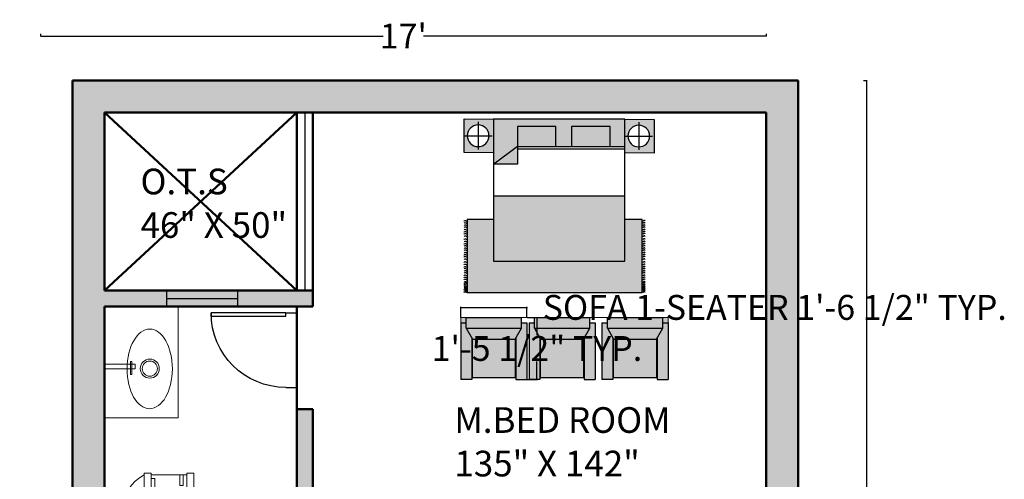
# Model space of a CAD drawing. Units: inches. Extents: x 679 to 1269, y 101 to 755.
# Tile 6 of 6: x 971 to 1248, y 626 to 755. Entities that reach past the tile are written whole.
import ezdxf

# ---------------------------------------------------------------- set-up
doc = ezdxf.new("R2010")
doc.units = ezdxf.units.IN
doc.header["$MEASUREMENT"] = 0
for name, color, linetype, lineweight in [('A-ANNO-DIMS', 2, 'Continuous', 18), ('A-AREA-IDEN', 7, 'Continuous', 25), ('A-DOOR', 4, 'Continuous', 25), ('A-FLOR-FIXT', 8, 'Continuous', 18), ('A-FURN', 32, 'Continuous', 18), ('A-FURN-PATT', 252, 'Continuous', 13), ('A-GLAZ', 4, 'Continuous', 25), ('A-WALL', 7, 'Continuous', 50), ('A-WALL-PATT', 8, 'Continuous', 13)]:
    doc.layers.add(name, color=color, linetype=linetype, lineweight=lineweight)
doc.layers.add('furniture', color=32, linetype='Continuous')
doc.styles.get("Standard").update_dxf_attribs({"font": 'arial.ttf'})
doc.dimstyles.get("Standard").update_dxf_attribs({"dimtxt": 7, "dimasz": 0.18, "dimexe": 0.18, "dimexo": 0.0625, "dimgap": 0.09, "dimtad": 0, "dimtih": 1, "dimtoh": 1, "dimzin": 0, "dimdsep": 46, "dimlunit": 3, "dimtxsty": 'Standard', "dimcen": 0.09, "dimadec": 0, "dimazin": 0, "dimtfac": 1, "dimtofl": 0, "dimtmove": 0, "dimatfit": 3, "dimfxl": 1, "dimtolj": 1, "dimtzin": 0, "dimarcsym": 0})

# ---------------------------------------------------------------- blocks, each defined once
blk = doc.blocks.new('*U4')
for p, q in [((0, 0), (0, -6)), ((40, 0), (40, -6))]:
    blk.add_line(p, q)
blk.add_lwpolyline([(0, 0), (0, 40), (1.75, 40), (1.75, 0)], close=True)
blk.add_arc((0, 0), 40, 0, 90)
blk = doc.blocks.new('CARPET')
at = {"layer": 'furniture'}
for p, q in [((-51.53, -98.11), (-51.53, -55.12)), ((-51.53, -55.12), (-41.27, -55.12)), ((36, -55.12), (51.55, -55.12)), ((51.55, -55.12), (51.55, -98.11)), ((51.55, -98.11), (-51.53, -98.11))]:
    blk.add_line(p, q, dxfattribs=at)
for points, knots in [([(-53.37, -55.99), (-53.22, -55.8), (-52.9, -55.41), (-52.34, -55.8), (-51.89, -56.08), (-51.65, -55.91), (-51.53, -55.83)], [0, 0, 0, 0, 0.653278, 1.290138, 1.740457, 2.114451, 2.114451, 2.114451, 2.114451]), ([(-53.37, -57.26), (-53.22, -57.07), (-52.9, -56.67), (-52.34, -57.07), (-51.89, -57.35), (-51.65, -57.17), (-51.53, -57.1)], [0, 0, 0, 0, 0.653278, 1.290138, 1.740457, 2.114451, 2.114451, 2.114451, 2.114451]), ([(53.37, -55.99), (53.22, -55.8), (52.9, -55.41), (52.34, -55.8), (51.89, -56.08), (51.65, -55.91), (51.53, -55.83)], [0, 0, 0, 0, 0.653278, 1.290138, 1.740457, 2.114451, 2.114451, 2.114451, 2.114451]), ([(53.37, -57.26), (53.22, -57.07), (52.9, -56.67), (52.34, -57.07), (51.89, -57.35), (51.65, -57.17), (51.53, -57.1)], [0, 0, 0, 0, 0.653278, 1.290138, 1.740457, 2.114451, 2.114451, 2.114451, 2.114451]), ([(-53.37, -58.59), (-53.22, -58.4), (-52.9, -58.01), (-52.34, -58.4), (-51.89, -58.68), (-51.65, -58.5), (-51.53, -58.43)], [0, 0, 0, 0, 0.653278, 1.290138, 1.740457, 2.114451, 2.114451, 2.114451, 2.114451]), ([(-53.37, -59.78), (-53.22, -59.58), (-52.9, -59.19), (-52.34, -59.58), (-51.89, -59.86), (-51.65, -59.69), (-51.53, -59.61)], [0, 0, 0, 0, 0.653278, 1.290138, 1.740457, 2.114451, 2.114451, 2.114451, 2.114451]), ([(-53.37, -61.22), (-53.22, -61.02), (-52.9, -60.63), (-52.34, -61.02), (-51.89, -61.3), (-51.65, -61.13), (-51.53, -61.05)], [0, 0, 0, 0, 0.653278, 1.290138, 1.740457, 2.114451, 2.114451, 2.114451, 2.114451]), ([(-53.37, -62.44), (-53.22, -62.25), (-52.9, -61.86), (-52.34, -62.25), (-51.89, -62.53), (-51.65, -62.36), (-51.53, -62.28)], [0, 0, 0, 0, 0.653278, 1.290138, 1.740457, 2.114451, 2.114451, 2.114451, 2.114451]), ([(-53.37, -63.63), (-53.22, -63.43), (-52.9, -63.04), (-52.34, -63.43), (-51.89, -63.72), (-51.65, -63.54), (-51.53, -63.46)], [0, 0, 0, 0, 0.653278, 1.290138, 1.740457, 2.114451, 2.114451, 2.114451, 2.114451]), ([(53.37, -58.59), (53.22, -58.4), (52.9, -58.01), (52.34, -58.4), (51.89, -58.68), (51.65, -58.5), (51.53, -58.43)], [0, 0, 0, 0, 0.653278, 1.290138, 1.740457, 2.114451, 2.114451, 2.114451, 2.114451]), ([(53.37, -59.78), (53.22, -59.58), (52.9, -59.19), (52.34, -59.58), (51.89, -59.86), (51.65, -59.69), (51.53, -59.61)], [0, 0, 0, 0, 0.653278, 1.290138, 1.740457, 2.114451, 2.114451, 2.114451, 2.114451]), ([(53.37, -61.22), (53.22, -61.02), (52.9, -60.63), (52.34, -61.02), (51.89, -61.3), (51.65, -61.13), (51.53, -61.05)], [0, 0, 0, 0, 0.653278, 1.290138, 1.740457, 2.114451, 2.114451, 2.114451, 2.114451]), ([(53.37, -62.44), (53.22, -62.25), (52.9, -61.86), (52.34, -62.25), (51.89, -62.53), (51.65, -62.36), (51.53, -62.28)], [0, 0, 0, 0, 0.653278, 1.290138, 1.740457, 2.114451, 2.114451, 2.114451, 2.114451]), ([(53.37, -63.63), (53.22, -63.43), (52.9, -63.04), (52.34, -63.43), (51.89, -63.72), (51.65, -63.54), (51.53, -63.46)], [0, 0, 0, 0, 0.653278, 1.290138, 1.740457, 2.114451, 2.114451, 2.114451, 2.114451]), ([(-53.37, -65.07), (-53.22, -64.87), (-52.9, -64.48), (-52.34, -64.87), (-51.89, -65.15), (-51.65, -64.98), (-51.53, -64.9)], [0, 0, 0, 0, 0.653278, 1.290138, 1.740457, 2.114451, 2.114451, 2.114451, 2.114451]), ([(-53.37, -66.76), (-53.22, -66.56), (-52.9, -66.17), (-52.34, -66.56), (-51.89, -66.84), (-51.65, -66.67), (-51.53, -66.59)], [0, 0, 0, 0, 0.653278, 1.290138, 1.740457, 2.114451, 2.114451, 2.114451, 2.114451]), ([(-53.37, -68.2), (-53.22, -68), (-52.9, -67.61), (-52.34, -68), (-51.89, -68.28), (-51.65, -68.11), (-51.53, -68.03)], [0, 0, 0, 0, 0.653278, 1.290138, 1.740457, 2.114451, 2.114451, 2.114451, 2.114451]), ([(-53.37, -69.53), (-53.22, -69.33), (-52.9, -68.94), (-52.34, -69.33), (-51.89, -69.61), (-51.65, -69.44), (-51.53, -69.36)], [0, 0, 0, 0, 0.653278, 1.290138, 1.740457, 2.114451, 2.114451, 2.114451, 2.114451]), ([(53.37, -65.07), (53.22, -64.87), (52.9, -64.48), (52.34, -64.87), (51.89, -65.15), (51.65, -64.98), (51.53, -64.9)], [0, 0, 0, 0, 0.653278, 1.290138, 1.740457, 2.114451, 2.114451, 2.114451, 2.114451]), ([(53.37, -66.76), (53.22, -66.56), (52.9, -66.17), (52.34, -66.56), (51.89, -66.84), (51.65, -66.67), (51.53, -66.59)], [0, 0, 0, 0, 0.653278, 1.290138, 1.740457, 2.114451, 2.114451, 2.114451, 2.114451]), ([(53.37, -68.2), (53.22, -68), (52.9, -67.61), (52.34, -68), (51.89, -68.28), (51.65, -68.11), (51.53, -68.03)], [0, 0, 0, 0, 0.653278, 1.290138, 1.740457, 2.114451, 2.114451, 2.114451, 2.114451]), ([(53.37, -69.53), (53.22, -69.33), (52.9, -68.94), (52.34, -69.33), (51.89, -69.61), (51.65, -69.44), (51.53, -69.36)], [0, 0, 0, 0, 0.653278, 1.290138, 1.740457, 2.114451, 2.114451, 2.114451, 2.114451]), ([(-53.37, -70.79), (-53.22, -70.6), (-52.9, -70.21), (-52.34, -70.6), (-51.89, -70.88), (-51.65, -70.7), (-51.53, -70.63)], [0, 0, 0, 0, 0.653278, 1.290138, 1.740457, 2.114451, 2.114451, 2.114451, 2.114451]), ([(-53.37, -72.12), (-53.22, -71.93), (-52.9, -71.54), (-52.34, -71.93), (-51.89, -72.21), (-51.65, -72.04), (-51.53, -71.96)], [0, 0, 0, 0, 0.653278, 1.290138, 1.740457, 2.114451, 2.114451, 2.114451, 2.114451]), ([(-53.37, -73.31), (-53.22, -73.11), (-52.9, -72.72), (-52.34, -73.11), (-51.89, -73.4), (-51.65, -73.22), (-51.53, -73.14)], [0, 0, 0, 0, 0.653278, 1.290138, 1.740457, 2.114451, 2.114451, 2.114451, 2.114451]), ([(-53.37, -74.75), (-53.22, -74.55), (-52.9, -74.16), (-52.34, -74.55), (-51.89, -74.83), (-51.65, -74.66), (-51.53, -74.58)], [0, 0, 0, 0, 0.653278, 1.290138, 1.740457, 2.114451, 2.114451, 2.114451, 2.114451]), ([(53.37, -70.79), (53.22, -70.6), (52.9, -70.21), (52.34, -70.6), (51.89, -70.88), (51.65, -70.7), (51.53, -70.63)], [0, 0, 0, 0, 0.653278, 1.290138, 1.740457, 2.114451, 2.114451, 2.114451, 2.114451]), ([(53.37, -72.12), (53.22, -71.93), (52.9, -71.54), (52.34, -71.93), (51.89, -72.21), (51.65, -72.04), (51.53, -71.96)], [0, 0, 0, 0, 0.653278, 1.290138, 1.740457, 2.114451, 2.114451, 2.114451, 2.114451]), ([(53.37, -73.31), (53.22, -73.11), (52.9, -72.72), (52.34, -73.11), (51.89, -73.4), (51.65, -73.22), (51.53, -73.14)], [0, 0, 0, 0, 0.653278, 1.290138, 1.740457, 2.114451, 2.114451, 2.114451, 2.114451]), ([(53.37, -74.75), (53.22, -74.55), (52.9, -74.16), (52.34, -74.55), (51.89, -74.83), (51.65, -74.66), (51.53, -74.58)], [0, 0, 0, 0, 0.653278, 1.290138, 1.740457, 2.114451, 2.114451, 2.114451, 2.114451]), ([(-53.37, -75.98), (-53.22, -75.78), (-52.9, -75.39), (-52.34, -75.78), (-51.89, -76.06), (-51.65, -75.89), (-51.53, -75.81)], [0, 0, 0, 0, 0.653278, 1.290138, 1.740457, 2.114451, 2.114451, 2.114451, 2.114451]), ([(-53.37, -77.16), (-53.22, -76.96), (-52.9, -76.57), (-52.34, -76.96), (-51.89, -77.25), (-51.65, -77.07), (-51.53, -76.99)], [0, 0, 0, 0, 0.653278, 1.290138, 1.740457, 2.114451, 2.114451, 2.114451, 2.114451]), ([(-53.37, -78.6), (-53.22, -78.4), (-52.9, -78.01), (-52.34, -78.4), (-51.89, -78.68), (-51.65, -78.51), (-51.53, -78.43)], [0, 0, 0, 0, 0.653278, 1.290138, 1.740457, 2.114451, 2.114451, 2.114451, 2.114451]), ([(-53.37, -80.29), (-53.22, -80.09), (-52.9, -79.7), (-52.34, -80.09), (-51.89, -80.37), (-51.65, -80.2), (-51.53, -80.12)], [0, 0, 0, 0, 0.653278, 1.290138, 1.740457, 2.114451, 2.114451, 2.114451, 2.114451]), ([(53.37, -75.98), (53.22, -75.78), (52.9, -75.39), (52.34, -75.78), (51.89, -76.06), (51.65, -75.89), (51.53, -75.81)], [0, 0, 0, 0, 0.653278, 1.290138, 1.740457, 2.114451, 2.114451, 2.114451, 2.114451]), ([(53.37, -77.16), (53.22, -76.96), (52.9, -76.57), (52.34, -76.96), (51.89, -77.25), (51.65, -77.07), (51.53, -76.99)], [0, 0, 0, 0, 0.653278, 1.290138, 1.740457, 2.114451, 2.114451, 2.114451, 2.114451]), ([(53.37, -78.6), (53.22, -78.4), (52.9, -78.01), (52.34, -78.4), (51.89, -78.68), (51.65, -78.51), (51.53, -78.43)], [0, 0, 0, 0, 0.653278, 1.290138, 1.740457, 2.114451, 2.114451, 2.114451, 2.114451]), ([(53.37, -80.29), (53.22, -80.09), (52.9, -79.7), (52.34, -80.09), (51.89, -80.37), (51.65, -80.2), (51.53, -80.12)], [0, 0, 0, 0, 0.653278, 1.290138, 1.740457, 2.114451, 2.114451, 2.114451, 2.114451]), ([(-53.37, -81.73), (-53.22, -81.53), (-52.9, -81.14), (-52.34, -81.53), (-51.89, -81.81), (-51.65, -81.64), (-51.53, -81.56)], [0, 0, 0, 0, 0.653278, 1.290138, 1.740457, 2.114451, 2.114451, 2.114451, 2.114451]), ([(-53.37, -83.06), (-53.22, -82.86), (-52.9, -82.47), (-52.34, -82.86), (-51.89, -83.14), (-51.65, -82.97), (-51.53, -82.89)], [0, 0, 0, 0, 0.653278, 1.290138, 1.740457, 2.114451, 2.114451, 2.114451, 2.114451]), ([(-53.37, -84.18), (-53.22, -83.99), (-52.9, -83.6), (-52.34, -83.99), (-51.89, -84.27), (-51.65, -84.09), (-51.53, -84.02)], [0, 0, 0, 0, 0.653278, 1.290138, 1.740457, 2.114451, 2.114451, 2.114451, 2.114451]), ([(-53.37, -85.51), (-53.22, -85.32), (-52.9, -84.93), (-52.34, -85.32), (-51.89, -85.6), (-51.65, -85.42), (-51.53, -85.35)], [0, 0, 0, 0, 0.653278, 1.290138, 1.740457, 2.114451, 2.114451, 2.114451, 2.114451]), ([(-53.37, -86.7), (-53.22, -86.5), (-52.9, -86.11), (-52.34, -86.5), (-51.89, -86.78), (-51.65, -86.61), (-51.53, -86.53)], [0, 0, 0, 0, 0.653278, 1.290138, 1.740457, 2.114451, 2.114451, 2.114451, 2.114451]), ([(53.37, -81.73), (53.22, -81.53), (52.9, -81.14), (52.34, -81.53), (51.89, -81.81), (51.65, -81.64), (51.53, -81.56)], [0, 0, 0, 0, 0.653278, 1.290138, 1.740457, 2.114451, 2.114451, 2.114451, 2.114451]), ([(53.37, -83.06), (53.22, -82.86), (52.9, -82.47), (52.34, -82.86), (51.89, -83.14), (51.65, -82.97), (51.53, -82.89)], [0, 0, 0, 0, 0.653278, 1.290138, 1.740457, 2.114451, 2.114451, 2.114451, 2.114451]), ([(53.37, -84.18), (53.22, -83.99), (52.9, -83.6), (52.34, -83.99), (51.89, -84.27), (51.65, -84.09), (51.53, -84.02)], [0, 0, 0, 0, 0.653278, 1.290138, 1.740457, 2.114451, 2.114451, 2.114451, 2.114451]), ([(53.37, -85.51), (53.22, -85.32), (52.9, -84.93), (52.34, -85.32), (51.89, -85.6), (51.65, -85.42), (51.53, -85.35)], [0, 0, 0, 0, 0.653278, 1.290138, 1.740457, 2.114451, 2.114451, 2.114451, 2.114451]), ([(53.37, -86.7), (53.22, -86.5), (52.9, -86.11), (52.34, -86.5), (51.89, -86.78), (51.65, -86.61), (51.53, -86.53)], [0, 0, 0, 0, 0.653278, 1.290138, 1.740457, 2.114451, 2.114451, 2.114451, 2.114451]), ([(-53.37, -88.14), (-53.22, -87.94), (-52.9, -87.55), (-52.34, -87.94), (-51.89, -88.22), (-51.65, -88.05), (-51.53, -87.97)], [0, 0, 0, 0, 0.653278, 1.290138, 1.740457, 2.114451, 2.114451, 2.114451, 2.114451]), ([(-53.37, -89.36), (-53.22, -89.17), (-52.9, -88.78), (-52.34, -89.17), (-51.89, -89.45), (-51.65, -89.28), (-51.53, -89.2)], [0, 0, 0, 0, 0.653278, 1.290138, 1.740457, 2.114451, 2.114451, 2.114451, 2.114451]), ([(-53.37, -90.55), (-53.22, -90.35), (-52.9, -89.96), (-52.34, -90.35), (-51.89, -90.64), (-51.65, -90.46), (-51.53, -90.38)], [0, 0, 0, 0, 0.653278, 1.290138, 1.740457, 2.114451, 2.114451, 2.114451, 2.114451]), ([(-53.37, -91.99), (-53.22, -91.79), (-52.9, -91.4), (-52.34, -91.79), (-51.89, -92.07), (-51.65, -91.9), (-51.53, -91.82)], [0, 0, 0, 0, 0.653278, 1.290138, 1.740457, 2.114451, 2.114451, 2.114451, 2.114451]), ([(-53.37, -92.69), (-53.22, -92.48), (-52.9, -92.08), (-52.35, -92.49), (-51.89, -92.77), (-51.65, -92.6), (-51.53, -92.52)], [0, 0, 0, 0, 0.663904, 1.307406, 1.757725, 2.131719, 2.131719, 2.131719, 2.131719]), ([(53.37, -88.14), (53.22, -87.94), (52.9, -87.55), (52.34, -87.94), (51.89, -88.22), (51.65, -88.05), (51.53, -87.97)], [0, 0, 0, 0, 0.653278, 1.290138, 1.740457, 2.114451, 2.114451, 2.114451, 2.114451]), ([(53.37, -89.36), (53.22, -89.17), (52.9, -88.78), (52.34, -89.17), (51.89, -89.45), (51.65, -89.28), (51.53, -89.2)], [0, 0, 0, 0, 0.653278, 1.290138, 1.740457, 2.114451, 2.114451, 2.114451, 2.114451]), ([(53.37, -90.55), (53.22, -90.35), (52.9, -89.96), (52.34, -90.35), (51.9, -90.63), (51.66, -90.47), (51.55, -90.4)], [0, 0, 0, 0, 0.653278, 1.290138, 1.740457, 2.0926, 2.0926, 2.0926, 2.0926]), ([(53.37, -91.99), (53.22, -91.79), (52.9, -91.4), (52.34, -91.79), (51.9, -92.07), (51.66, -91.91), (51.55, -91.83)], [0, 0, 0, 0, 0.653278, 1.290138, 1.740457, 2.0926, 2.0926, 2.0926, 2.0926]), ([(53.37, -92.69), (53.22, -92.49), (52.9, -92.09), (52.34, -92.49), (51.9, -92.77), (51.66, -92.61), (51.55, -92.53)], [0, 0, 0, 0, 0.656792, 1.295826, 1.746145, 2.098292, 2.098292, 2.098292, 2.098292]), ([(-53.37, -93.61), (-53.22, -93.42), (-52.9, -93.03), (-52.34, -93.42), (-51.89, -93.7), (-51.65, -93.52), (-51.53, -93.45)], [0, 0, 0, 0, 0.653278, 1.290138, 1.740457, 2.114451, 2.114451, 2.114451, 2.114451]), ([(-53.37, -94.55), (-53.22, -94.35), (-52.9, -93.96), (-52.34, -94.35), (-51.89, -94.63), (-51.65, -94.46), (-51.53, -94.38)], [0, 0, 0, 0, 0.653278, 1.290138, 1.740457, 2.114451, 2.114451, 2.114451, 2.114451]), ([(-53.37, -95.05), (-53.22, -94.85), (-52.9, -94.46), (-52.34, -94.85), (-51.89, -95.14), (-51.65, -94.96), (-51.53, -94.88)], [0, 0, 0, 0, 0.653278, 1.290138, 1.740457, 2.114451, 2.114451, 2.114451, 2.114451]), ([(-53.37, -95.73), (-53.22, -95.54), (-52.9, -95.15), (-52.34, -95.54), (-51.89, -95.82), (-51.65, -95.65), (-51.53, -95.57)], [0, 0, 0, 0, 0.653278, 1.290138, 1.740457, 2.114451, 2.114451, 2.114451, 2.114451]), ([(-53.37, -96.38), (-53.22, -96.18), (-52.9, -95.79), (-52.34, -96.18), (-51.89, -96.47), (-51.65, -96.29), (-51.53, -96.21)], [0, 0, 0, 0, 0.653278, 1.290138, 1.740457, 2.114451, 2.114451, 2.114451, 2.114451]), ([(-53.37, -97.17), (-53.22, -96.98), (-52.9, -96.59), (-52.34, -96.98), (-51.89, -97.26), (-51.65, -97.08), (-51.53, -97.01)], [0, 0, 0, 0, 0.653278, 1.290138, 1.740457, 2.114451, 2.114451, 2.114451, 2.114451]), ([(-53.37, -97.99), (-53.22, -97.79), (-52.9, -97.4), (-52.34, -97.79), (-51.89, -98.08), (-51.65, -97.9), (-51.53, -97.82)], [0, 0, 0, 0, 0.653278, 1.290138, 1.740457, 2.114451, 2.114451, 2.114451, 2.114451]), ([(53.37, -95.78), (53.22, -95.58), (52.9, -95.19), (52.34, -95.58), (51.89, -95.86), (51.65, -95.69), (51.53, -95.61)], [0, 0, 0, 0, 0.653278, 1.290138, 1.740457, 2.114451, 2.114451, 2.114451, 2.114451]), ([(53.37, -96.43), (53.22, -96.23), (52.9, -95.84), (52.34, -96.23), (51.89, -96.51), (51.65, -96.34), (51.53, -96.26)], [0, 0, 0, 0, 0.653278, 1.290138, 1.740457, 2.114451, 2.114451, 2.114451, 2.114451]), ([(53.37, -97.22), (53.22, -97.02), (52.9, -96.63), (52.34, -97.02), (51.89, -97.3), (51.65, -97.13), (51.53, -97.05)], [0, 0, 0, 0, 0.653278, 1.290138, 1.740457, 2.114451, 2.114451, 2.114451, 2.114451]), ([(53.37, -97.99), (53.22, -97.79), (52.9, -97.4), (52.34, -97.79), (51.89, -98.08), (51.65, -97.9), (51.53, -97.82)], [0, 0, 0, 0, 0.653278, 1.290138, 1.740457, 2.114451, 2.114451, 2.114451, 2.114451]), ([(53.37, -93.66), (53.22, -93.46), (52.9, -93.07), (52.34, -93.46), (51.9, -93.74), (51.66, -93.58), (51.55, -93.5)], [0, 0, 0, 0, 0.653278, 1.290138, 1.740457, 2.0926, 2.0926, 2.0926, 2.0926]), ([(53.37, -94.59), (53.22, -94.4), (52.9, -94.01), (52.34, -94.4), (51.9, -94.68), (51.66, -94.51), (51.55, -94.44)], [0, 0, 0, 0, 0.653278, 1.290138, 1.740457, 2.0926, 2.0926, 2.0926, 2.0926]), ([(53.37, -95.1), (53.22, -94.9), (52.9, -94.51), (52.34, -94.9), (51.9, -95.18), (51.66, -95.02), (51.55, -94.94)], [0, 0, 0, 0, 0.653278, 1.290138, 1.740457, 2.0926, 2.0926, 2.0926, 2.0926])]:
    blk.add_open_spline(points, degree=3, knots=knots, dxfattribs=at)
blk = doc.blocks.new('A$C58D270C6')
at = {"layer": 'furniture'}
for p, q in [((9.09, 124.13), (9.09, 108.87)), ((1.46, 116.5), (16.73, 116.5)), ((14.97, 94.84), (24.62, 107.92)), ((24.62, 94.93), (24.62, 107.92)), ((42.08, 108), (42.08, 36)), ((14.97, 94.93), (24.62, 94.93)), ((14.97, 94.84), (14.97, 36)), ((16.22, 94.93), (16.22, 36)), ((9.25, 36), (9.25, 20.74)), ((1.62, 28.37), (16.88, 28.37))]:
    blk.add_line(p, q, dxfattribs=at)
for points in [[(18.5, 108), (18.34, 124.13), (-0.16, 124.13), (0, 108)], [(0, 108), (77.91, 108), (77.91, 36), (0, 36)], [(4.09, 94.93), (14.97, 94.93), (14.97, 73.83), (4.09, 73.83)], [(4.09, 65.23), (14.97, 65.23), (14.97, 44.13), (4.09, 44.13)], [(18.65, 19.87), (18.5, 36), (0, 36), (0.16, 19.87)]]:
    blk.add_lwpolyline(points, close=True, dxfattribs=at)
for centre in [(9.09, 116.5), (9.25, 28.37)]:
    blk.add_circle(centre, 5.95, dxfattribs=at)
at = {"layer": 'furniture', "xscale": 0.9312884925094044, "yscale": 0.9312884925094044, "zscale": 0.9312884925094044, "rotation": 90}
blk.add_blockref('CARPET', (3.79, 74.47), dxfattribs=at)
blk = doc.blocks.new('FABRIC SOFA 1S')
at = {"layer": 'furniture'}
for p, q in [((3, 18.12), (34, 18.12)), ((3, 15.12), (3, 18.12)), ((34, 12.12), (34, 18.12)), ((0, -15.12), (0, 15.12)), ((6, 15.12), (0, 15.12)), ((6, -15.12), (6, 15.12)), ((12, 11.75), (6, 15.12)), ((11.33, 12.12), (34, 12.12)), ((6, -15.12), (0, -15.12)), ((3, -18.12), (3, -15.12)), ((6, -15.12), (12, -11.75)), ((11.33, -12.12), (34, -12.12)), ((34, -12.12), (34, -18.12)), ((3, -18.12), (34, -18.12))]:
    blk.add_line(p, q, dxfattribs=at)
blk.add_lwpolyline([(12, -11.75), (12, 11.75), (33, 11.75), (33, -11.75)], close=True, dxfattribs=at)
blk = doc.blocks.new('*U12')
for p, q in [((-10, 22), (-10, 12)), ((-10, 21), (-7, 21)), ((-7, 20), (-10, 20)), ((-7, 21), (-7, 20)), ((10, 12), (10, 22)), ((10.5, 12), (-10.5, 12)), ((-10.5, 10), (-10.5, 12)), ((9, 13), (-9, 13)), ((-9, 13), (-9, 12)), ((9, 12), (9, 13)), ((10.5, 12), (10.5, 10)), ((10.5, 10), (-10.5, 10)), ((-3, 4.4065), (-3, 2)), ((-2, 2), (-2, 4.1658)), ((2, 4.1658), (2, 2)), ((3, 2), (3, 4.4065)), ((4, 2), (-4, 2)), ((-4, 2), (-4, 1)), ((4, 1), (4, 2))]:
    blk.add_line(p, q)
for points in [[(10.5, 22), (10.5, 24), (-10.5, 24), (-10.5, 22)], [(6, 0), (6, 1), (-6, 1), (-6, 0)]]:
    blk.add_lwpolyline(points, close=True)
blk.add_arc((0, 15.3333), 11.3333, 208.0725, 331.9275)
blk = doc.blocks.new('*D15')
at = {"layer": 'A-ANNO-DIMS', "color": 0, "lineweight": -2, "transparency": 16777216}
for p, q in [((976.93, 750.86), (976.93, 750.04)), ((1180.93, 750.86), (1180.93, 750.04)), ((977.11, 750.22), (1073.23, 750.22)), ((1180.75, 750.22), (1084.63, 750.22))]:
    blk.add_line(p, q, dxfattribs=at)
at = {"layer": 'A-ANNO-DIMS', "color": 0, "transparency": 16777216}
for points in [[(977.11, 750.25), (977.11, 750.19), (976.93, 750.22)], [(1180.75, 750.25), (1180.75, 750.19), (1180.93, 750.22)]]:
    blk.add_solid(points, dxfattribs=at)
at = {"layer": 'Defpoints', "color": 0, "transparency": 16777216}
for p in [(976.93, 750.92), (1180.93, 750.92), (1180.93, 750.22)]:
    blk.add_point(p, dxfattribs=at)
at = {"layer": 'A-ANNO-DIMS', "color": 0, "transparency": 16777216, "insert": (1078.93, 750.22), "char_height": 7, "attachment_point": 5}
blk.add_mtext("\\A1;17'", dxfattribs=at)
blk = doc.blocks.new('*D16')
at = {"layer": 'A-ANNO-DIMS', "color": 0, "lineweight": -2, "transparency": 16777216}
for p, q in [((1208.37, 737.73), (1209.33, 737.73)), ((1209.15, 737.55), (1209.15, 441.39)), ((1209.15, 137.91), (1209.15, 434.07)), ((1208.37, 137.73), (1209.33, 137.73))]:
    blk.add_line(p, q, dxfattribs=at)
at = {"layer": 'A-ANNO-DIMS', "color": 0, "transparency": 16777216}
for points in [[(1209.12, 737.55), (1209.18, 737.55), (1209.15, 737.73)], [(1209.12, 137.91), (1209.18, 137.91), (1209.15, 137.73)]]:
    blk.add_solid(points, dxfattribs=at)
at = {"layer": 'Defpoints', "color": 0, "transparency": 16777216}
for p in [(1208.3, 737.73), (1208.3, 137.73), (1209.15, 137.73)]:
    blk.add_point(p, dxfattribs=at)
at = {"layer": 'A-ANNO-DIMS', "color": 0, "transparency": 16777216, "insert": (1209.15, 437.73), "char_height": 7, "attachment_point": 5}
blk.add_mtext("\\A1;50'", dxfattribs=at)
blk = doc.blocks.new('WASHBASIN')
for p, q in [((8.57, 12.49), (0, 12.49)), ((8.57, 11.25), (0, 11.25)), ((7.24, 9.62), (7.23, 13.28)), ((7.23, 13.28), (7.63, 13.28)), ((7.63, 13.28), (7.65, 9.63)), ((8.57, 11.25), (8.57, 12.49)), ((7.24, 9.62), (7.65, 9.63))]:
    blk.add_line(p, q)
for radius in [2.67, 2.13]:
    blk.add_circle((12.7, 11.27), radius)
at = {"extrusion": (0, 0, -1)}
blk.add_ellipse((12.66, 11.2), major_axis=(0.03, 11.2), ratio=0.56899, dxfattribs=at)
blk = doc.blocks.new('*D25')
at = {"layer": 'A-ANNO-DIMS', "color": 0, "lineweight": -2, "transparency": 16777216}
for p, q in [((1095.05, 671.2), (1095.05, 674.12)), ((1095.23, 673.94), (1113.51, 673.94)), ((1113.69, 671.2), (1113.69, 674.12)), ((1113.69, 673.94), (1113.87, 673.94))]:
    blk.add_line(p, q, dxfattribs=at)
at = {"layer": 'A-ANNO-DIMS', "color": 0, "transparency": 16777216}
for points in [[(1095.23, 673.97), (1095.23, 673.91), (1095.05, 673.94)], [(1113.51, 673.97), (1113.51, 673.91), (1113.69, 673.94)]]:
    blk.add_solid(points, dxfattribs=at)
at = {"layer": 'Defpoints', "color": 0, "transparency": 16777216}
for p in [(1113.69, 673.94), (1095.05, 671.14), (1113.69, 671.14)]:
    blk.add_point(p, dxfattribs=at)
at = {"layer": 'A-ANNO-DIMS', "color": 0, "transparency": 16777216, "insert": (1183.37, 673.94), "char_height": 7, "attachment_point": 5}
blk.add_mtext('\\A1;SOFA 1-SEATER 1\'-6 1/2" TYP.', dxfattribs=at)
blk = doc.blocks.new('*D26')
at = {"layer": 'A-ANNO-DIMS', "color": 0, "lineweight": -2, "transparency": 16777216}
for p, q in [((1113.75, 671.14), (1116.67, 671.14)), ((1116.49, 670.96), (1116.49, 666.11)), ((1116.49, 653.84), (1116.49, 658.69)), ((1113.75, 653.66), (1116.67, 653.66))]:
    blk.add_line(p, q, dxfattribs=at)
at = {"layer": 'A-ANNO-DIMS', "color": 0, "transparency": 16777216}
for points in [[(1116.46, 670.96), (1116.52, 670.96), (1116.49, 671.14)], [(1116.46, 653.84), (1116.52, 653.84), (1116.49, 653.66)]]:
    blk.add_solid(points, dxfattribs=at)
at = {"layer": 'Defpoints', "color": 0, "transparency": 16777216}
for p in [(1113.69, 671.14), (1113.69, 653.66), (1116.49, 653.66)]:
    blk.add_point(p, dxfattribs=at)
at = {"layer": 'A-ANNO-DIMS', "color": 0, "transparency": 16777216, "insert": (1116.49, 662.4), "char_height": 7, "attachment_point": 5}
blk.add_mtext('\\A1;1\'-5 1/2" TYP.', dxfattribs=at)

msp = doc.modelspace()

# ---------------------------------------------------------------- hatches: boundary and pattern name
at = {"layer": 'A-FURN-PATT'}
h = msp.add_hatch(color=256, dxfattribs=at)
h.dxf.hatch_style = 1
h.paths.add_polyline_path([(1141.204, 705.293), (1104.314, 705.293), (1104.314, 686.937), (1141.204, 686.937)])
h.paths.add_polyline_path([(1121.819, 724.754), (1111.01, 724.754), (1111.01, 719.18), (1121.819, 719.18)], flags=17)
h.paths.add_polyline_path([(1137.038, 724.754), (1126.229, 724.754), (1126.229, 719.18), (1137.038, 719.18)], flags=17)
h.paths.add_polyline_path([(1111.01, 724.754), (1121.819, 724.754), (1121.819, 719.18), (1126.229, 719.18), (1126.229, 724.754), (1137.038, 724.754), (1137.038, 719.18), (1141.204, 719.18), (1141.204, 726.852), (1104.314, 726.852), (1104.314, 714.239), (1104.354, 714.239), (1111.01, 719.147)])
h = msp.add_hatch(color=256, dxfattribs=at)
h.dxf.hatch_style = 1
h.paths.add_polyline_path([(1111.01, 719.147), (1104.354, 714.239), (1111.01, 714.239)])
h.paths.add_polyline_path([(1146.082, 698.607), (1141.204, 698.607), (1141.204, 686.937), (1104.314, 686.937), (1104.314, 698.607), (1096.893, 698.607), (1096.893, 678.097), (1146.082, 678.097)])
h = msp.add_hatch(color=256, dxfattribs=at)
h.dxf.hatch_style = 1
h.paths.add_polyline_path([(1112.147, 671.141), (1096.592, 671.141), (1096.592, 668.056), (1112.147, 668.056)])
h.paths.add_polyline_path([(1096.592, 671.141), (1095.05, 671.141), (1095.05, 669.599), (1096.592, 669.599)])
h.paths.add_polyline_path([(1098.135, 665.313), (1096.592, 668.056), (1096.592, 669.599), (1095.05, 669.599), (1095.05, 653.658), (1098.135, 653.658)])
h.paths.add_polyline_path([(1113.69, 669.599), (1112.147, 669.599), (1112.147, 668.056), (1110.605, 665.313), (1110.605, 653.658), (1113.69, 653.658)])
h.paths.add_polyline_path([(1112.147, 668.056), (1096.592, 668.056), (1098.328, 664.971), (1110.412, 664.971)])
h.paths.add_polyline_path([(1110.412, 664.971), (1098.328, 664.971), (1098.328, 654.172), (1110.412, 654.172)])
h = msp.add_hatch(color=256, dxfattribs=at)
h.dxf.hatch_style = 1
h.paths.add_polyline_path([(1131.356, 671.141), (1115.801, 671.141), (1115.801, 668.056), (1131.356, 668.056)])
h.paths.add_polyline_path([(1117.343, 665.313), (1115.801, 668.056), (1115.801, 669.599), (1114.258, 669.599), (1114.258, 653.658), (1117.343, 653.658)])
h.paths.add_polyline_path([(1132.898, 669.599), (1131.356, 669.599), (1131.356, 668.056), (1129.813, 665.313), (1129.813, 653.658), (1132.898, 653.658)])
h.paths.add_polyline_path([(1131.356, 668.056), (1115.801, 668.056), (1117.536, 664.971), (1129.62, 664.971)])
h.paths.add_polyline_path([(1129.62, 664.971), (1117.536, 664.971), (1117.536, 654.172), (1129.62, 654.172)])
h = msp.add_hatch(color=256, dxfattribs=at)
h.dxf.hatch_style = 1
h.paths.add_polyline_path([(1137.85, 665.313), (1136.307, 668.056), (1136.307, 669.599), (1134.765, 669.599), (1134.765, 653.658), (1137.85, 653.658)])
h.paths.add_polyline_path([(1151.862, 671.141), (1136.307, 671.141), (1136.307, 668.056), (1151.862, 668.056)])
h.paths.add_polyline_path([(1153.405, 671.141), (1151.862, 671.141), (1151.862, 669.599), (1153.405, 669.599)])
h.paths.add_polyline_path([(1151.862, 668.056), (1136.307, 668.056), (1138.043, 664.971), (1150.127, 664.971)])
h.paths.add_polyline_path([(1153.405, 669.599), (1151.862, 669.599), (1151.862, 668.056), (1150.32, 665.313), (1150.32, 653.658), (1153.405, 653.658)])
h = msp.add_hatch(color=256, dxfattribs=at)
h.dxf.hatch_style = 1
h.paths.add_polyline_path([(1150.127, 664.971), (1138.043, 664.971), (1138.043, 654.172), (1150.127, 654.172)])
at = {"layer": 'A-GLAZ'}
h = msp.add_hatch(color=256, dxfattribs=at)
h.dxf.hatch_style = 1
h.paths.add_polyline_path([(994.931, 583.729), (1053.502, 583.729), (1053.502, 588.883), (1053.502, 623.243), (1053.502, 645.329), (1049.002, 645.329), (1049.002, 588.229), (994.931, 588.229), (994.931, 674.229), (1053.502, 674.229), (1053.502, 678.729), (994.931, 678.729), (994.931, 728.729), (1180.931, 728.729), (1180.931, 356.354), (1033.405, 356.354), (1033.405, 351.854), (1119.805, 351.854), (1119.805, 281.2), (1124.305, 281.2), (1124.305, 351.854), (1180.931, 351.854), (1180.931, 251.542), (1161.199, 251.542), (1161.199, 247.042), (1189.931, 247.042), (1189.931, 737.729), (985.931, 737.729), (985.931, 137.729), (1015.759, 137.729), (1015.759, 146.729), (994.931, 146.729)])
h.paths.add_polyline_path([(1185.698, 247.042), (1180.931, 247.042), (1180.931, 146.729), (1124.305, 146.729), (1124.305, 142.229), (1185.698, 142.229)], flags=0)
h.paths.add_polyline_path([(1189.931, 247.042), (1185.698, 247.042), (1185.698, 142.229), (1124.305, 142.229), (1124.305, 137.729), (1189.931, 137.729)], flags=17)
at = {"layer": 'A-WALL-PATT'}
h = msp.add_hatch(color=256, dxfattribs=at)
h.dxf.hatch_style = 1
h.paths.add_polyline_path([(1189.931, 737.729), (985.931, 737.729), (985.931, 137.729), (1015.759, 137.729), (1015.759, 146.729), (994.931, 146.729), (994.931, 583.729), (1053.502, 583.729), (1053.502, 645.329), (1049.002, 645.329), (1049.002, 588.229), (994.931, 588.229), (994.931, 674.229), (1012.305, 674.229), (1012.305, 678.729), (994.931, 678.729), (994.931, 728.729), (1053.502, 728.729), (1053.502, 678.729), (1053.502, 674.229), (1049.002, 674.229), (1049.002, 645.329), (1053.502, 645.329), (1053.502, 583.729), (994.931, 583.729), (994.931, 146.729), (1180.931, 146.729), (1180.931, 247.042), (1124.305, 247.042), (1124.305, 176.159), (1119.805, 176.159), (1119.805, 181.227), (1104.539, 181.227), (1104.539, 251.542), (1119.805, 251.542), (1124.238, 251.542), (1124.238, 281.2), (1119.805, 281.2), (1119.805, 331.601), (1036.785, 331.601), (1036.785, 351.854), (1033.393, 351.854), (1033.393, 356.354), (1033.405, 356.354), (1089.362, 356.354), (1089.362, 507.268), (1180.931, 507.268), (1180.931, 356.354), (1089.362, 356.354), (1033.405, 356.354), (1033.405, 351.854), (1119.805, 351.854), (1119.805, 281.2), (1124.305, 281.2), (1124.305, 351.854), (1180.931, 351.854), (1180.931, 251.542), (1161.199, 251.542), (1161.199, 247.042), (1189.931, 247.042)], flags=17)
h.paths.add_polyline_path([(1087.931, 548.661), (1087.931, 583.729), (1087.862, 588.229), (1087.862, 583.729), (1087.931, 583.729), (1150.34, 583.729), (1150.34, 548.661)], flags=0)
h.paths.add_polyline_path([(1161.61, 599.984, -0.2489628), (1161.61, 610.804), (1161.61, 612.705, -0.611129), (1176.66, 612.705), (1176.66, 610.804, -0.2489628), (1176.66, 599.984)], flags=0)
h.paths.add_polyline_path([(1064.382, 534.011), (1064.382, 508.83), (1050.613, 508.83), (1050.613, 534.011)], flags=0)
h.paths.add_polyline_path([(1153.405, 653.658), (1150.32, 653.658), (1150.32, 654.172), (1137.85, 654.172), (1137.85, 653.658), (1134.765, 653.658), (1134.765, 669.599), (1136.307, 669.599), (1136.307, 671.141), (1131.356, 671.141), (1131.356, 669.599), (1132.898, 669.599), (1132.898, 653.658), (1129.813, 653.658), (1129.813, 654.172), (1117.343, 654.172), (1117.343, 653.658), (1114.258, 653.658), (1114.258, 669.599), (1115.801, 669.599), (1115.801, 671.141), (1112.147, 671.141), (1112.147, 669.599), (1113.69, 669.599), (1113.69, 653.658), (1110.605, 653.658), (1110.605, 654.172), (1098.135, 654.172), (1098.135, 653.658), (1095.05, 653.658), (1095.05, 669.599), (1095.05, 671.141), (1096.592, 671.141), (1112.147, 671.141), (1115.801, 671.141), (1131.356, 671.141), (1136.307, 671.141), (1151.862, 671.141), (1153.405, 671.141), (1153.405, 669.599)], flags=0)
h.paths.add_polyline_path([(1037.949, 548.144), (1037.949, 541.332), (1012.214, 541.332), (1012.971, 540.906), (1036.813, 540.906), (1036.813, 432.764), (1012.971, 432.764), (1006.159, 428.933), (999.347, 428.933), (999.347, 544.738), (1002.753, 544.738), (1002.753, 548.144)], flags=0)
h.paths.add_polyline_path([(1037.949, 550.347), (999.347, 550.347), (999.347, 579.213), (1037.949, 579.213)], flags=0)
h.paths.add_polyline_path([(1064.382, 465.7), (1064.382, 440.519), (1050.613, 440.519), (1050.613, 465.7)], flags=0)
h.paths.add_polyline_path([(1146.082, 678.097), (1096.893, 678.097), (1096.893, 698.607), (1104.314, 698.607), (1104.314, 717.374), (1096.049, 717.453), (1096.049, 726.931), (1104.314, 726.852), (1141.204, 726.852), (1149.469, 726.772), (1149.469, 717.294), (1141.204, 717.374), (1141.204, 698.607), (1146.082, 698.607)], flags=0)
h.paths.add_polyline_path([(1189.931, 737.729), (985.931, 737.729), (985.931, 137.729), (1015.759, 137.729), (1015.759, 146.729), (994.931, 146.729), (994.931, 583.729), (1053.502, 583.729), (1053.502, 645.329), (1049.002, 645.329), (1049.002, 588.229), (994.931, 588.229), (994.931, 674.229), (1012.305, 674.229), (1012.305, 678.729), (994.931, 678.729), (994.931, 728.729), (1053.502, 728.729), (1053.502, 674.229), (1049.002, 674.229), (1049.002, 645.329), (1053.502, 645.329), (1053.502, 583.729), (994.931, 583.729), (994.931, 146.729), (1180.931, 146.729), (1180.931, 247.042), (1124.305, 247.042), (1124.305, 176.159), (1119.805, 176.159), (1119.805, 181.227), (1104.539, 181.227), (1104.539, 251.542), (1119.805, 251.542), (1124.238, 251.542), (1124.238, 281.2), (1119.805, 281.2), (1119.805, 331.601), (1036.785, 331.601), (1036.785, 351.854), (1033.393, 351.854), (1033.393, 356.354), (1089.362, 356.354), (1089.362, 507.268), (1180.931, 507.268), (1180.931, 356.354), (1033.405, 356.354), (1033.405, 351.854), (1119.805, 351.854), (1119.805, 281.2), (1124.305, 281.2), (1124.305, 351.854), (1180.931, 351.854), (1180.931, 251.542), (1161.199, 251.542), (1161.199, 247.042), (1189.931, 247.042)], flags=17)
h.paths.add_polyline_path([(1087.931, 583.729), (1087.862, 583.729), (1087.862, 588.229), (1087.862, 588.883), (1087.862, 596.11), (1152.762, 596.11), (1158.171, 599.984), (1161.61, 599.984, -0.2489628), (1161.61, 610.804), (1161.61, 612.705, -0.611129), (1176.66, 612.705), (1176.66, 610.804, -0.2489628), (1176.66, 599.984), (1161.61, 599.984), (1158.171, 599.984), (1152.762, 596.11), (1087.862, 596.11), (1087.862, 588.883), (1087.862, 588.229), (1087.931, 583.729), (1150.34, 583.729), (1150.34, 548.661), (1087.931, 548.661)], flags=0)
h.paths.add_polyline_path([(1087.931, 583.729), (1087.862, 588.229), (1087.862, 583.729), (1150.34, 583.729), (1150.34, 548.661), (1087.931, 548.661)], flags=0)
h.paths.add_polyline_path([(1161.61, 610.804), (1161.61, 612.705, -0.611129), (1176.66, 612.705), (1176.66, 610.804, -0.2489628), (1176.66, 599.984), (1176.66, 610.804, 0.4904831), (1161.61, 610.804), (1161.61, 599.984, -0.2489628)], flags=0)
h = msp.add_hatch(color=256, dxfattribs=at)
h.dxf.hatch_style = 1
h.paths.add_polyline_path([(1180.931, 507.268), (1089.362, 507.268), (1089.362, 356.354), (1180.931, 356.354)])
h.paths.add_polyline_path([(1037.949, 416.536), (999.347, 416.536), (999.347, 387.67), (1037.949, 387.67)])
h.paths.add_polyline_path([(1037.949, 579.213), (999.347, 579.213), (999.347, 550.347), (1037.949, 550.347)])
h.paths.add_polyline_path([(1064.382, 465.7), (1050.613, 465.7), (1050.613, 440.519), (1064.382, 440.519)])
h.paths.add_polyline_path([(1064.382, 534.011), (1050.613, 534.011), (1050.613, 508.83), (1064.382, 508.83)])
h.paths.add_polyline_path([(1017.114, 194.268), (1003.506, 194.268), (1003.391, 182.402), (1010.195, 182.402), (1010.195, 183.635, -0.4142136), (1005.815, 188.015, -1), (1014.576, 188.015, -0.4142136), (1010.195, 183.635), (1010.195, 182.402), (1017, 182.402)])
h.paths.add_polyline_path([(1014.691, 252.849, -0.4142136), (1010.31, 248.468), (1010.31, 247.235), (1017.114, 247.235), (1017.229, 259.102), (1003.62, 259.102), (1003.506, 247.235), (1010.31, 247.235), (1010.31, 248.468, -0.4142136), (1005.929, 252.849, -1)])
h.paths.add_polyline_path([(1104.314, 726.852), (1096.049, 726.931), (1096.049, 722.192), (1096.908, 722.192, -1), (1103.01, 722.192, -1), (1096.908, 722.192), (1096.049, 722.192), (1096.049, 717.453), (1104.314, 717.374)])
h.paths.add_polyline_path([(1149.469, 726.772), (1141.204, 726.852), (1141.204, 722.113), (1142.063, 722.113, -1), (1148.165, 722.113, -1), (1142.063, 722.113), (1141.204, 722.113), (1141.204, 717.374), (1149.469, 717.294)])
h.paths.add_polyline_path([(826.598, 726.852), (818.333, 726.931), (818.333, 722.192), (819.192, 722.192, -1), (825.294, 722.192, -1), (819.192, 722.192), (818.333, 722.192), (818.333, 717.453), (826.598, 717.374)])
h.paths.add_polyline_path([(871.752, 726.772), (863.487, 726.852), (863.487, 722.113), (864.346, 722.113, -1), (870.448, 722.113, -1), (864.346, 722.113), (863.487, 722.113), (863.487, 717.374), (871.752, 717.294)])

# ---------------------------------------------------------------- linework, layer by layer
at = {"layer": 'A-FLOR-FIXT'}
for p, q in [((1015.607, 674.229), (1015.607, 642.902)), ((1015.607, 642.902), (994.931, 642.902))]:
    msp.add_line(p, q, dxfattribs=at)
at = {"layer": 'A-FURN'}
for p, q in [((1096.592, 671.141), (1095.05, 671.141)), ((1095.05, 671.141), (1095.05, 669.599)), ((1112.147, 671.141), (1115.801, 671.141)), ((1115.801, 671.141), (1136.307, 671.141)), ((1136.307, 671.141), (1153.405, 671.141)), ((1153.405, 669.599), (1153.405, 671.141))]:
    msp.add_line(p, q, dxfattribs=at)
at = {"layer": 'A-GLAZ'}
for p, q in [((1049.002, 728.729), (1049.002, 678.729)), ((1051.252, 728.729), (1051.252, 678.729)), ((1053.502, 678.729), (1053.502, 728.729)), ((1032.249, 678.729), (1012.305, 678.729)), ((1012.305, 678.729), (1012.305, 674.229)), ((1032.249, 678.729), (1032.249, 674.229)), ((1012.305, 676.479), (1032.249, 676.479)), ((1012.305, 674.229), (1032.249, 674.229))]:
    msp.add_line(p, q, dxfattribs=at)
at = {"layer": 'A-WALL'}
for p, q in [((985.931, 737.729), (1189.931, 737.729)), ((985.931, 137.729), (985.931, 737.729)), ((1189.931, 737.729), (1189.931, 137.729)), ((994.931, 728.729), (1180.931, 728.729)), ((994.931, 728.729), (1049.002, 678.729)), ((994.931, 678.729), (1049.002, 728.729)), ((994.931, 678.729), (994.931, 728.729)), ((1049.002, 678.729), (1049.002, 728.729)), ((1049.002, 678.729), (1049.002, 728.729)), ((1053.502, 674.229), (1053.502, 728.729)), ((1053.502, 674.229), (1053.502, 728.729)), ((1180.931, 728.729), (1180.931, 356.354)), ((994.931, 678.729), (1053.502, 678.729)), ((994.931, 674.229), (1053.502, 674.229)), ((994.931, 588.229), (994.931, 674.229)), ((1049.002, 588.229), (1049.002, 674.229)), ((1053.502, 645.329), (1049.002, 645.329)), ((1053.502, 583.729), (1053.502, 645.329))]:
    msp.add_line(p, q, dxfattribs=at)

# ---------------------------------------------------------------- block references
at = {"layer": 'A-DOOR', "xscale": -0.524704002908781, "yscale": 0.524704002908781, "zscale": 0.524704002908781, "rotation": 90}
msp.add_blockref('*U4', (1045.854, 672.403), dxfattribs=at)
at = {"layer": 'A-FLOR-FIXT'}
msp.add_blockref('WASHBASIN', (994.931, 645.451), dxfattribs=at)
at = {"layer": 'A-FLOR-FIXT', "rotation": 269.9999999999999}
msp.add_blockref('*U12', (996.046, 616.875), dxfattribs=at)
at = {"layer": 'A-FURN'}
for name, p, xscale, yscale, zscale, rotation in [('A$C58D270C6', (1159.649, 726.852), -0.5123565564710688, 0.5123565564710688, 0.5123565564710688, 90), ('FABRIC SOFA 1S', (1104.37, 671.141), 0.5142158862385126, 0.5142158862385126, 0.5142158862385126, 270), ('FABRIC SOFA 1S', (1123.578, 671.141), 0.5142158862385126, 0.5142158862385126, 0.5142158862385126, 270), ('FABRIC SOFA 1S', (1144.085, 671.141), 0.5142158862385126, 0.5142158862385126, 0.5142158862385126, 270)]:
    msp.add_blockref(name, p, dxfattribs=dict(at, xscale=xscale, yscale=yscale, zscale=zscale, rotation=rotation))

# ---------------------------------------------------------------- texts
at = {"layer": 'A-AREA-IDEN'}
for s, height, p in [('O.T.S', 7.213, (1005.011, 705.725)), ('46" X 50"', 7.213, (1005.011, 693.485)), ('M.BED ROOM', 7.213, (1093.271, 638.667)), ('135" X 142"', 7.21303, (1093.271, 626.427))]:
    msp.add_text(s, height=height, dxfattribs=at).set_placement(p)

# ---------------------------------------------------------------- dimensions: what is measured, and where the dimension line sits
at = {"layer": 'A-ANNO-DIMS'}
dim = msp.add_linear_dim(base=(1180.931, 750.216), p1=(976.931, 750.921), p2=(1180.931, 750.921), dimstyle='Standard', override={"dimclrd": 0, "dimclre": 0, "dimclrt": 0}, dxfattribs=at)
dim.commit()
dim.dimension.update_dxf_attribs({"geometry": '*D15', "text_midpoint": (1078.931, 750.216)})
dim = msp.add_linear_dim(base=(1209.153, 137.729), p1=(1208.303, 737.729), p2=(1208.303, 137.729), angle=90, dimstyle='Standard', override={"dimclrd": 0, "dimclre": 0, "dimclrt": 0}, dxfattribs=at)
dim.commit()
dim.dimension.update_dxf_attribs({"geometry": '*D16', "text_midpoint": (1209.153, 437.729)})
dim = msp.add_linear_dim(base=(1113.69, 673.937), p1=(1095.05, 671.141), p2=(1113.69, 671.141), text='SOFA 1-SEATER <> TYP.', dimstyle='Standard', override={"dimdec": 1, "dimrnd": 0, "dimzin": 1, "dimlunit": 4, "dimfrac": 2}, dxfattribs=at)
dim.commit()
dim.dimension.update_dxf_attribs({"geometry": '*D25', "text_midpoint": (1183.373, 673.937)})
dim = msp.add_linear_dim(base=(1116.486, 653.658), p1=(1113.69, 671.141), p2=(1113.69, 653.658), angle=270, text='<> TYP.', dimstyle='Standard', override={"dimdec": 1, "dimrnd": 0, "dimzin": 1, "dimlunit": 4, "dimfrac": 2}, dxfattribs=at)
dim.commit()
dim.dimension.update_dxf_attribs({"geometry": '*D26', "text_midpoint": (1116.486, 662.4)})

doc.saveas('drawing.dxf')
